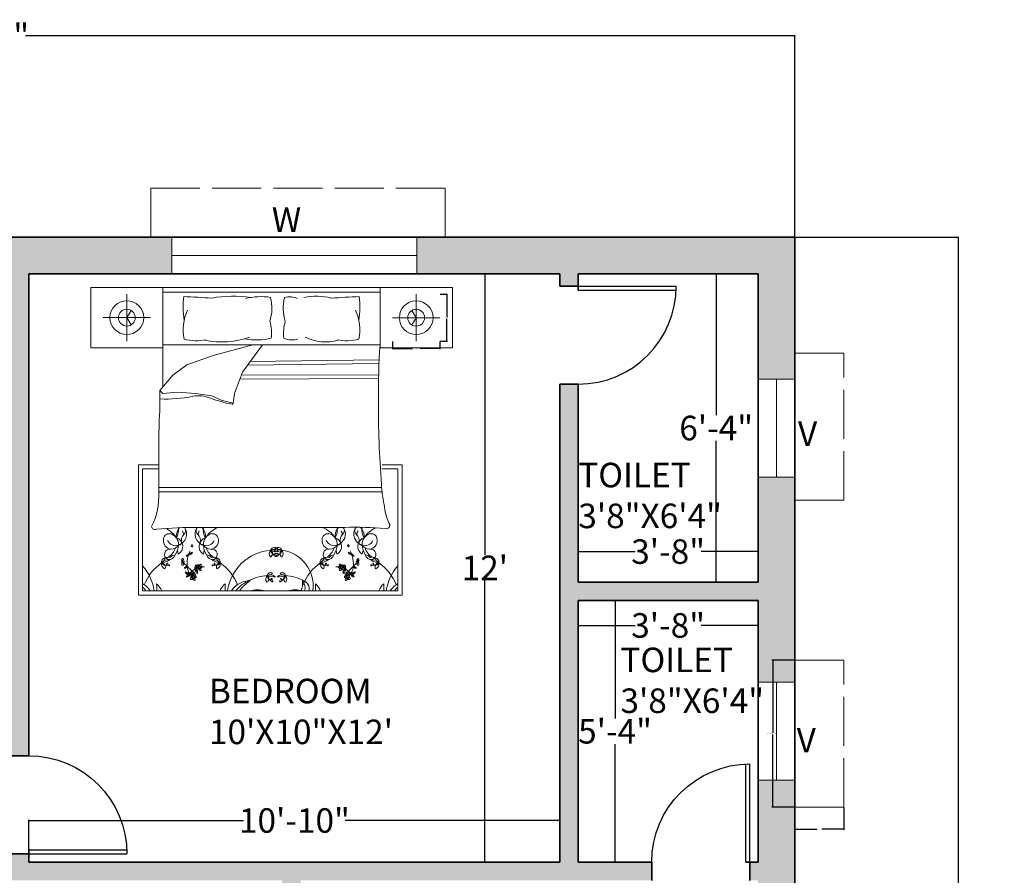
# Model space of a CAD drawing. Units: inches. Extents: x -5 to 482, y -460 to 66.
# Tile 31 of 31: x 241 to 482, y -143 to 66. Entities that reach past the tile are written whole.
import ezdxf

# ---------------------------------------------------------------- set-up
doc = ezdxf.new("R2010")
doc.units = ezdxf.units.IN
doc.header["$MEASUREMENT"] = 0
doc.linetypes.add('ACAD_ISO02W100', pattern=[15, 12, -3])
for name, color, linetype, lineweight in [('A-ANNO-DIMS', 2, 'Continuous', 18), ('A-ANNO-TEXT', 7, 'Continuous', 18), ('A-AREA-IDEN', 7, 'Continuous', 18), ('A-DOOR', 3, 'Continuous', 25), ('A-FURN', 8, 'Continuous', 18), ('A-GLAZ', 4, 'Continuous', 18), ('A-GLAZ-OVHD', 4, 'ACAD_ISO02W100', 13), ('A-WALL', 7, 'Continuous', 35), ('A-WALL-PATT', 152, 'Continuous', 13)]:
    doc.layers.add(name, color=color, linetype=linetype, lineweight=lineweight)
doc.styles.get("Standard").update_dxf_attribs({"font": 'arial.ttf'})
doc.dimstyles.get("Standard").update_dxf_attribs({"dimtxt": 0.18, "dimasz": 0.18, "dimexe": 0.18, "dimexo": 0.0625, "dimgap": 0.09, "dimtad": 0, "dimtih": 1, "dimtoh": 1, "dimdec": 0, "dimzin": 0, "dimdsep": 46, "dimlunit": 3, "dimtxsty": 'Standard', "dimcen": 0.09, "dimadec": 0, "dimazin": 0, "dimtfac": 1, "dimtdec": 0, "dimtofl": 0, "dimtmove": 0, "dimatfit": 3, "dimfxl": 1, "dimtolj": 1, "dimtzin": 0, "dimarcsym": 0})

# ---------------------------------------------------------------- blocks, each defined once
blk = doc.blocks.new('*D3')
at = {"layer": 'A-ANNO-DIMS', "color": 0, "lineweight": -2, "transparency": 16777216}
for p, q in [((32.88, 13.21), (32.88, 62.61)), ((33.06, 62.43), (221.23, 62.43)), ((430.2, 62.43), (242.02, 62.43)), ((430.38, 13.21), (430.38, 62.61))]:
    blk.add_line(p, q, dxfattribs=at)
at = {"layer": 'A-ANNO-DIMS', "color": 0, "transparency": 16777216}
for points in [[(33.06, 62.46), (33.06, 62.4), (32.88, 62.43)], [(430.2, 62.46), (430.2, 62.4), (430.38, 62.43)]]:
    blk.add_solid(points, dxfattribs=at)
at = {"layer": 'Defpoints', "color": 0, "transparency": 16777216}
for p in [(430.38, 62.43), (32.88, 13.15), (430.38, 13.15)]:
    blk.add_point(p, dxfattribs=at)
at = {"layer": 'A-ANNO-DIMS', "color": 0, "transparency": 16777216, "insert": (231.63, 62.43), "char_height": 6, "attachment_point": 5}
blk.add_mtext('\\A1;33\'-2"', dxfattribs=at)
blk = doc.blocks.new('*D4')
at = {"layer": 'A-ANNO-DIMS', "color": 0, "lineweight": -2, "transparency": 16777216}
for p, q in [((430.44, 13.15), (470.55, 13.15)), ((470.37, 12.97), (470.37, -201.19)), ((470.37, -421.67), (470.37, -207.5)), ((430.44, -421.85), (470.55, -421.85))]:
    blk.add_line(p, q, dxfattribs=at)
at = {"layer": 'A-ANNO-DIMS', "color": 0, "transparency": 16777216}
for points in [[(470.34, 12.97), (470.4, 12.97), (470.37, 13.15)], [(470.34, -421.67), (470.4, -421.67), (470.37, -421.85)]]:
    blk.add_solid(points, dxfattribs=at)
at = {"layer": 'Defpoints', "color": 0, "transparency": 16777216}
for p in [(430.38, 13.15), (430.38, -421.85), (470.37, -421.85)]:
    blk.add_point(p, dxfattribs=at)
at = {"layer": 'A-ANNO-DIMS', "color": 0, "transparency": 16777216, "insert": (470.37, -204.35), "char_height": 6, "attachment_point": 5}
blk.add_mtext('\\A1;36\'-3"', dxfattribs=at)
blk = doc.blocks.new('*D9')
at = {"layer": 'A-ANNO-DIMS', "color": 0, "lineweight": -2, "transparency": 16777216}
for p, q in [((242.88, -137.79), (242.88, -129.51)), ((243.06, -129.69), (295.43, -129.69)), ((372.7, -129.69), (320.32, -129.69)), ((372.88, -129.63), (372.88, -129.51))]:
    blk.add_line(p, q, dxfattribs=at)
at = {"layer": 'A-ANNO-DIMS', "color": 0, "transparency": 16777216}
for points in [[(243.06, -129.66), (243.06, -129.72), (242.88, -129.69)], [(372.7, -129.66), (372.7, -129.72), (372.88, -129.69)]]:
    blk.add_solid(points, dxfattribs=at)
at = {"layer": 'Defpoints', "color": 0, "transparency": 16777216}
for p in [(372.88, -129.69), (372.88, -129.69), (242.88, -137.85)]:
    blk.add_point(p, dxfattribs=at)
at = {"layer": 'A-ANNO-DIMS', "color": 0, "transparency": 16777216, "insert": (307.88, -129.69), "char_height": 6, "attachment_point": 5}
blk.add_mtext('\\A1;10\'-10"', dxfattribs=at)
blk = doc.blocks.new('*D10')
at = {"layer": 'A-ANNO-DIMS', "color": 0, "lineweight": -2, "transparency": 16777216}
for p, q in [((355.37, 4.15), (354.32, 4.15)), ((354.5, 3.97), (354.5, -64.75)), ((354.5, -139.67), (354.5, -70.95)), ((355.37, -139.85), (354.32, -139.85))]:
    blk.add_line(p, q, dxfattribs=at)
at = {"layer": 'A-ANNO-DIMS', "color": 0, "transparency": 16777216}
for points in [[(354.47, 3.97), (354.53, 3.97), (354.5, 4.15)], [(354.47, -139.67), (354.53, -139.67), (354.5, -139.85)]]:
    blk.add_solid(points, dxfattribs=at)
at = {"layer": 'Defpoints', "color": 0, "transparency": 16777216}
for p in [(355.43, 4.15), (354.5, -139.85), (355.43, -139.85)]:
    blk.add_point(p, dxfattribs=at)
at = {"layer": 'A-ANNO-DIMS', "color": 0, "transparency": 16777216, "insert": (354.5, -67.85), "char_height": 6, "attachment_point": 5}
blk.add_mtext("\\A1;12'", dxfattribs=at)
blk = doc.blocks.new('*D11')
at = {"layer": 'A-ANNO-DIMS', "color": 0, "lineweight": -2, "transparency": 16777216}
for p, q in [((377.38, -63.79), (377.38, -63.67)), ((377.56, -63.85), (391.31, -63.85)), ((421.2, -63.85), (407.44, -63.85)), ((421.38, -63.79), (421.38, -63.67))]:
    blk.add_line(p, q, dxfattribs=at)
at = {"layer": 'A-ANNO-DIMS', "color": 0, "transparency": 16777216}
for points in [[(377.56, -63.82), (377.56, -63.88), (377.38, -63.85)], [(421.2, -63.82), (421.2, -63.88), (421.38, -63.85)]]:
    blk.add_solid(points, dxfattribs=at)
at = {"layer": 'Defpoints', "color": 0, "transparency": 16777216}
for p in [(377.38, -63.85), (421.38, -63.85), (421.38, -63.85)]:
    blk.add_point(p, dxfattribs=at)
at = {"layer": 'A-ANNO-DIMS', "color": 0, "transparency": 16777216, "insert": (399.38, -63.85), "char_height": 6, "attachment_point": 5}
blk.add_mtext('\\A1;3\'-8"', dxfattribs=at)
blk = doc.blocks.new('*D12')
at = {"layer": 'A-ANNO-DIMS', "color": 0, "lineweight": -2, "transparency": 16777216}
for p, q in [((417.62, 4.15), (410.96, 4.15)), ((411.14, 3.97), (411.14, -30.45)), ((411.14, -71.17), (411.14, -36.75)), ((417.62, -71.35), (410.96, -71.35))]:
    blk.add_line(p, q, dxfattribs=at)
at = {"layer": 'A-ANNO-DIMS', "color": 0, "transparency": 16777216}
for points in [[(411.11, 3.97), (411.17, 3.97), (411.14, 4.15)], [(411.11, -71.17), (411.17, -71.17), (411.14, -71.35)]]:
    blk.add_solid(points, dxfattribs=at)
at = {"layer": 'Defpoints', "color": 0, "transparency": 16777216}
for p in [(411.14, 4.15), (417.69, 4.15), (417.69, -71.35)]:
    blk.add_point(p, dxfattribs=at)
at = {"layer": 'A-ANNO-DIMS', "color": 0, "transparency": 16777216, "insert": (411.14, -33.6), "char_height": 6, "attachment_point": 5}
blk.add_mtext('\\A1;6\'-4"', dxfattribs=at)
blk = doc.blocks.new('*D13')
at = {"layer": 'A-ANNO-DIMS', "color": 0, "lineweight": -2, "transparency": 16777216}
for p, q in [((377.38, -81.87), (377.38, -81.75)), ((377.56, -81.93), (391.31, -81.93)), ((421.2, -81.93), (407.44, -81.93)), ((421.38, -81.87), (421.38, -81.75))]:
    blk.add_line(p, q, dxfattribs=at)
at = {"layer": 'A-ANNO-DIMS', "color": 0, "transparency": 16777216}
for points in [[(377.56, -81.9), (377.56, -81.96), (377.38, -81.93)], [(421.2, -81.9), (421.2, -81.96), (421.38, -81.93)]]:
    blk.add_solid(points, dxfattribs=at)
at = {"layer": 'Defpoints', "color": 0, "transparency": 16777216}
for p in [(377.38, -81.93), (421.38, -81.93), (421.38, -81.93)]:
    blk.add_point(p, dxfattribs=at)
at = {"layer": 'A-ANNO-DIMS', "color": 0, "transparency": 16777216, "insert": (399.38, -81.93), "char_height": 6, "attachment_point": 5}
blk.add_mtext('\\A1;3\'-8"', dxfattribs=at)
blk = doc.blocks.new('*D14')
at = {"layer": 'A-ANNO-DIMS', "color": 0, "lineweight": -2, "transparency": 16777216}
for p, q in [((382.91, -75.85), (386.56, -75.85)), ((386.38, -76.03), (386.38, -104.71)), ((386.38, -139.67), (386.38, -110.99)), ((386.44, -139.85), (386.56, -139.85))]:
    blk.add_line(p, q, dxfattribs=at)
at = {"layer": 'A-ANNO-DIMS', "color": 0, "transparency": 16777216}
for points in [[(386.35, -76.03), (386.41, -76.03), (386.38, -75.85)], [(386.35, -139.67), (386.41, -139.67), (386.38, -139.85)]]:
    blk.add_solid(points, dxfattribs=at)
at = {"layer": 'Defpoints', "color": 0, "transparency": 16777216}
for p in [(382.85, -75.85), (386.38, -75.85), (386.38, -139.85)]:
    blk.add_point(p, dxfattribs=at)
at = {"layer": 'A-ANNO-DIMS', "color": 0, "transparency": 16777216, "insert": (386.38, -107.85), "char_height": 6, "attachment_point": 5}
blk.add_mtext('\\A1;5\'-4"', dxfattribs=at)
blk = doc.blocks.new('DOOR-SWING-24IN')
for p, q in [((24, 1), (0, 1)), ((24, 0), (0, 0))]:
    blk.add_line(p, q)
blk.add_arc((24, 0), 24, 90, 180)
blk = doc.blocks.new('WIN-GLAZ-60IN')
for p, q in [((0, 9), (60, 9)), ((0, 4.5), (60, 4.5)), ((60, 0), (0, 0))]:
    blk.add_line(p, q)
blk = doc.blocks.new('VENT-GLAZ-24IN')
for p, q in [((0, 9), (24, 9)), ((0, 4.5), (24, 4.5)), ((24, 0), (0, 0))]:
    blk.add_line(p, q)
blk = doc.blocks.new('WIN-SHADE-72IN')
for p, q in [((0, 12), (72, 12)), ((0, 12), (0, 0)), ((72, 12), (72, 0))]:
    blk.add_line(p, q)
blk = doc.blocks.new('VENT-SHADE-36IN')
for p, q in [((0, 0), (0, 12)), ((36, 0), (36, 12)), ((0, 0), (36, 0))]:
    blk.add_line(p, q)
blk = doc.blocks.new('BEDSIDE-LAMP-8IN')
for p, q in [((5.79, 0), (5.79, 11.57)), ((0, 5.78), (11.57, 5.78))]:
    blk.add_line(p, q)
for points in [[(5.79, 5.78), (4.75, 7.57)], [(5.79, 5.78), (4.75, 4)]]:
    blk.add_lwpolyline(points)
for radius in [4.13, 2.07]:
    blk.add_circle((5.79, 5.78), radius)
blk = doc.blocks.new('*D51')
at = {"layer": 'A-ANNO-DIMS', "color": 0, "lineweight": -2, "transparency": 16777216}
for p, q in [((430.31, -90.42), (424.8, -90.42)), ((424.98, -90.6), (424.98, -108.23)), ((424.98, -126.24), (424.98, -108.6)), ((430.31, -126.42), (424.8, -126.42))]:
    blk.add_line(p, q, dxfattribs=at)
at = {"layer": 'A-ANNO-DIMS', "color": 0, "transparency": 16777216}
for points in [[(424.95, -90.6), (425.01, -90.6), (424.98, -90.42)], [(424.95, -126.24), (425.01, -126.24), (424.98, -126.42)]]:
    blk.add_solid(points, dxfattribs=at)
at = {"layer": 'Defpoints', "color": 0, "transparency": 16777216}
for p in [(424.98, -90.42), (430.38, -90.42), (430.38, -126.42)]:
    blk.add_point(p, dxfattribs=at)
at = {"layer": 'A-ANNO-DIMS', "color": 0, "transparency": 16777216, "insert": (424.98, -108.42), "char_height": 0.18, "attachment_point": 5}
blk.add_mtext('\\A1;VENT SHADE 3\'-0" TYP.', dxfattribs=at)
blk = doc.blocks.new('*D52')
at = {"layer": 'A-ANNO-DIMS', "color": 0, "lineweight": -2, "transparency": 16777216}
for p, q in [((430.38, -126.48), (430.38, -132)), ((442.38, -126.48), (442.38, -132)), ((430.56, -131.82), (435.75, -131.82)), ((442.2, -131.82), (437.01, -131.82))]:
    blk.add_line(p, q, dxfattribs=at)
at = {"layer": 'A-ANNO-DIMS', "color": 0, "transparency": 16777216}
for points in [[(430.56, -131.79), (430.56, -131.85), (430.38, -131.82)], [(442.2, -131.79), (442.2, -131.85), (442.38, -131.82)]]:
    blk.add_solid(points, dxfattribs=at)
at = {"layer": 'Defpoints', "color": 0, "transparency": 16777216}
for p in [(430.38, -126.42), (442.38, -126.42), (430.38, -131.82)]:
    blk.add_point(p, dxfattribs=at)
at = {"layer": 'A-ANNO-DIMS', "color": 0, "transparency": 16777216, "insert": (436.38, -131.82), "char_height": 0.18, "attachment_point": 5}
blk.add_mtext('\\A1;1\'-0" TYP.', dxfattribs=at)
blk = doc.blocks.new('*D55')
at = {"layer": 'A-ANNO-DIMS', "color": 0, "lineweight": -2, "transparency": 16777216}
for p, q in [((343.54, -0.8), (345.39, -0.8)), ((345.21, -0.98), (345.21, -6.4)), ((345.21, -12.19), (345.21, -6.77)), ((343.54, -12.37), (345.39, -12.37))]:
    blk.add_line(p, q, dxfattribs=at)
at = {"layer": 'A-ANNO-DIMS', "color": 0, "transparency": 16777216}
for points in [[(345.18, -0.98), (345.24, -0.98), (345.21, -0.8)], [(345.18, -12.19), (345.24, -12.19), (345.21, -12.37)]]:
    blk.add_solid(points, dxfattribs=at)
at = {"layer": 'Defpoints', "color": 0, "transparency": 16777216}
for p in [(343.48, -0.8), (345.21, -0.8), (343.48, -12.37)]:
    blk.add_point(p, dxfattribs=at)
at = {"layer": 'A-ANNO-DIMS', "color": 0, "transparency": 16777216, "insert": (345.21, -6.58), "char_height": 0.18, "attachment_point": 5}
blk.add_mtext('\\A1;BEDSIDE LAMP 0\'-11 1/2" TYP.', dxfattribs=at)
blk = doc.blocks.new('*D56')
at = {"layer": 'A-ANNO-DIMS', "color": 0, "lineweight": -2, "transparency": 16777216}
for p, q in [((331.91, -12.43), (331.91, -14.28)), ((332.09, -14.1), (336.78, -14.1)), ((343.3, -14.1), (338.61, -14.1)), ((343.48, -12.43), (343.48, -14.28))]:
    blk.add_line(p, q, dxfattribs=at)
at = {"layer": 'A-ANNO-DIMS', "color": 0, "transparency": 16777216}
for points in [[(332.09, -14.07), (332.09, -14.13), (331.91, -14.1)], [(343.3, -14.07), (343.3, -14.13), (343.48, -14.1)]]:
    blk.add_solid(points, dxfattribs=at)
at = {"layer": 'Defpoints', "color": 0, "transparency": 16777216}
for p in [(331.91, -12.37), (343.48, -12.37), (343.48, -14.1)]:
    blk.add_point(p, dxfattribs=at)
at = {"layer": 'A-ANNO-DIMS', "color": 0, "transparency": 16777216, "insert": (337.69, -14.1), "char_height": 0.18, "attachment_point": 5}
blk.add_mtext('\\A1;0\'-11 1/2" TYP.', dxfattribs=at)

msp = doc.modelspace()

# ---------------------------------------------------------------- hatches: boundary and pattern name
at = {"layer": 'A-WALL-PATT'}
h = msp.add_hatch(color=256, dxfattribs=at)
h.dxf.hatch_style = 1
h.paths.add_polyline_path([(149.38, -412.85), (144.38, -412.85), (144.38, -283.85), (144.38, -279.35), (133.88, -279.35), (133.88, -283.85), (139.88, -283.85), (139.88, -412.85), (133.51, -412.85), (133.51, -413.92), (102.65, -413.92), (102.65, -421.02), (133.51, -421.02), (133.51, -421.85), (149.38, -421.85)])
h.paths.add_polyline_path([(226.05, -412.85), (218.88, -412.85), (218.88, -350.85), (262.88, -350.85), (262.88, -386.85), (267.38, -386.85), (267.38, -283.85), (270.38, -283.85), (270.38, -279.35), (244.88, -279.35), (244.88, -283.85), (262.88, -283.85), (262.88, -346.35), (218.88, -346.35), (218.88, -283.85), (220.88, -283.85), (220.88, -279.35), (214.38, -279.35), (214.38, -283.85), (214.38, -412.85), (209.38, -412.85), (209.38, -421.85), (226.05, -421.85)])
h.paths.add_polyline_path([(315.81, -412.85), (250.05, -412.85), (250.05, -421.85), (315.81, -421.85)])
h.paths.add_polyline_path([(430.38, -378.35), (421.38, -378.35), (421.38, -412.85), (375.81, -412.85), (375.81, -421.85), (430.38, -421.85)])
h.paths.add_polyline_path([(78.69, -413.92), (47.68, -413.92), (47.68, -412.85), (41.88, -412.85), (41.88, -283.85), (109.88, -283.85), (109.88, -279.35), (41.88, -279.35), (41.88, -241.85), (32.88, -241.85), (32.88, -421.85), (47.68, -421.85), (47.68, -421.02), (78.69, -421.02)])
h.paths.add_polyline_path([(41.88, -144.35), (154.38, -144.35), (154.38, -137.85), (149.88, -137.85), (149.88, -139.85), (41.88, -139.85), (41.88, -97.85), (32.88, -97.85), (32.88, -181.85), (41.88, -181.85)])
h.paths.add_polyline_path([(430.38, -241.85), (421.38, -241.85), (421.38, -279.35), (309.38, -279.35), (309.38, -170.35), (304.88, -170.35), (304.88, -279.35), (294.38, -279.35), (294.38, -283.85), (421.38, -283.85), (421.38, -318.35), (430.38, -318.35)])
h.paths.add_polyline_path([(430.38, -119.85), (421.38, -119.85), (421.38, -139.85), (419.38, -139.85), (419.38, -144.35), (421.38, -144.35), (421.38, -181.85), (430.38, -181.85)])
h.paths.add_polyline_path([(395.38, -139.85), (377.38, -139.85), (377.38, -75.85), (421.38, -75.85), (421.38, -95.85), (430.38, -95.85), (430.38, -45.6), (421.38, -45.6), (421.38, -71.35), (377.38, -71.35), (377.38, -22.85), (372.88, -22.85), (372.88, -139.85), (242.88, -139.85), (242.88, -137.85), (238.38, -137.85), (238.38, -144.35), (304.88, -144.35), (304.88, -146.35), (309.38, -146.35), (309.38, -144.35), (395.38, -144.35)])
h.paths.add_polyline_path([(65.88, 13.15), (32.88, 13.15), (32.88, -37.85), (41.88, -37.85), (41.88, 4.15), (65.88, 4.15)])
h.paths.add_polyline_path([(166.38, 13.15), (125.88, 13.15), (125.88, 4.15), (149.88, 4.15), (149.88, -113.85), (154.38, -113.85), (154.38, 4.15), (166.38, 4.15)])
h.paths.add_polyline_path([(277.88, 13.15), (226.38, 13.15), (226.38, 4.15), (238.38, 4.15), (238.38, -113.85), (242.88, -113.85), (242.88, 4.15), (277.88, 4.15)])
h.paths.add_polyline_path([(430.38, 13.15), (337.88, 13.15), (337.88, 4.15), (372.88, 4.15), (372.88, 1.15), (377.38, 1.15), (377.38, 4.15), (421.38, 4.15), (421.38, -21.6), (430.38, -21.6)])

# ---------------------------------------------------------------- linework, layer by layer
at = {"layer": 'A-FURN'}
for p, q in [((258.01, 0.8), (346.55, 0.8)), ((275.71, 0.8), (275.71, -23.51)), ((328.84, -0.34), (275.71, -0.34)), ((275.71, -13.2), (328.84, -13.2)), ((288.01, -15.83), (297.67, -13.2)), ((300.04, -13.2), (295.19, -19.95)), ((281.56, -18.16), (288.01, -15.83)), ((278.15, -20.67), (281.56, -18.16)), ((328.57, -17.78), (296.42, -18.24)), ((328.6, -16.87), (297.08, -17.32)), ((274.92, -24.43), (278.15, -20.67)), ((295.19, -19.95), (293.21, -25.15)), ((328.53, -21.48), (294.55, -21.62)), ((328.52, -20.57), (294.9, -20.7)), ((275.64, -25.15), (274.92, -24.43)), ((279.23, -24.79), (275.64, -25.15)), ((283.71, -25.15), (279.23, -24.79)), ((287.65, -25.68), (283.71, -25.15)), ((289.99, -26.76), (287.65, -25.68)), ((293.21, -25.15), (292.86, -27.48)), ((292.86, -27.48), (289.99, -26.76)), ((269.69, -42.61), (274.7, -42.61)), ((269.69, -74.5), (269.69, -42.61)), ((329.33, -42.61), (334.24, -42.61)), ((334.24, -42.61), (334.24, -74.5)), ((274.7, -43.63), (270.72, -43.63)), ((270.72, -43.63), (270.72, -73.48)), ((333.22, -43.63), (329.31, -43.63)), ((333.22, -73.48), (333.22, -43.63)), ((329.24, -48.13), (274.69, -48.13)), ((329.33, -49.23), (274.69, -49.23)), ((320.25, -57.93), (284.3, -57.93)), ((279.44, -64.5), (279.25, -63.5)), ((285.63, -64.5), (285.83, -63.5)), ((318.3, -64.5), (318.11, -63.5)), ((324.49, -64.5), (324.69, -63.5)), ((334.24, -74.5), (269.69, -74.5)), ((270.72, -73.48), (333.22, -73.48))]:
    msp.add_line(p, q, dxfattribs=at)
for points in [[(275.71, -13.96), (258.01, -13.96), (258.01, 0.8)], [(328.84, 0.8), (328.84, -13.96), (346.55, -13.96), (346.55, 0.8)]]:
    msp.add_lwpolyline(points, dxfattribs=at)
for points in [[(280.8, -1.41, 0.074897), (280.91, -7.19, -0.472817)], [(301.86, -7.52, 0.14099), (302.04, -1.62, 0.235245)], [(305.64, -7.52, -0.14099), (305.47, -1.62, -0.235245)], [(323.75, -1.41, -0.074897), (323.65, -7.19, 0.472817)], [(274.74, -32.54, 0.001242), (274.69, -49.34, -0.127202), (272.92, -57.71)], [(329.22, -47.43, 0.056112), (329.86, -52.3, 0.095341), (331.1, -57)]]:
    msp.add_lwpolyline(points, format="xyb", dxfattribs=at)
for centre in [(284.56, -67.71), (319.38, -67.71), (283.08, -70.09), (320.85, -70.09)]:
    msp.add_circle(centre, 0.225, dxfattribs=at)
for centre, radius, start, end in [((329.6, 841.22), 844.04, 266.68521, 267.14978), ((292.93, -33.45), 32.11, 82.2196, 99.497), ((299.71, -17.22), 15.78, 81.5249, 103.96), ((306.68, -5.83), 4.38, 63.3437, 106.1026), ((313.25, -16.9), 15.57, 76.3427, 101.1841), ((274.95, 841.22), 844.04, 272.85022, 273.31479), ((292.08, -9.52), 11.41, 155.1316, 191.7583), ((312.47, -9.52), 11.41, 348.2417, 24.8684), ((291.43, -10.48), 10.85, 354.0129, 15.8293), ((316.08, -10.48), 10.85, 164.1707, 185.9871), ((283.96, -0.37), 11.87, 255.1039, 281.0369), ((290.2, 8.06), 20.58, 258.0397, 289.2615), ((298.54, 3.57), 15.61, 259.8617, 283.6238), ((307.27, -7.35), 4.69, 245.0183, 288.5407), ((315.47, -1.25), 11.27, 243.8761, 286.1746), ((320.6, -0.37), 11.87, 258.9631, 284.8961), ((487.57, -24.02), 159.1, 176.1, 180.9282), ((193.74, -26.63), 81.21, 355.8294, 1.553), ((276.44, 6.92), 33.42, 267.4519, 281.3392), ((284.42, -32.91), 7.21, 66.2616, 101.3392), ((299, 5.98), 34.34, 250.1194, 259.3383), ((292.65, -27.55), 0.214, 268.8623, 19.7536), ((536, -29.8), 207.53, 179.1145, 184.8735), ((273.73, -57.65), 0.817, 183.98, 297.3412), ((330.43, -57.45), 0.807, 246.5219, 33.8264), ((283.25, -150.1), 92.17, 89.3433, 95.6887), ((277.29, -60.95), 1.49, 84.4856, 181.0538), ((273.39, -64.17), 6.7, 33.6671, 63.2997), ((276.83, -62.05), 2.66, 355.2933, 76.921), ((282.37, -60.18), 3.41, 145.785, 184.7304), ((275.85, -58.59), 3.67, 328.8218, 9.1554), ((280.39, -58.91), 1.07, 120.0293, 142.325), ((278.69, -59.54), 2.82, 289.2822, 29.1751), ((282.02, -61.05), 1.82, 131.5653, 195.1471), ((278.26, -60.05), 2.55, 7.436, 29.9149), ((279.94, -58.7), 1.32, 311.5653, 23.8354), ((280.39, -58.91), 1.07, 44.4517, 63.558), ((286.39, -59.54), 2.82, 150.8249, 250.7178), ((285.14, -58.7), 1.32, 156.1646, 228.4347), ((284.69, -58.91), 1.07, 113.229, 135.5483), ((283.05, -61.05), 1.82, 344.8529, 48.4347), ((286.81, -60.05), 2.55, 150.0851, 172.564), ((284.69, -58.91), 1.07, 37.675, 66.7144), ((282.71, -60.18), 3.41, 355.2696, 34.215), ((289.23, -58.59), 3.67, 169.7133, 211.1782), ((288.24, -62.05), 2.66, 103.079, 184.7067), ((291.69, -64.17), 6.7, 111.4941, 146.3329), ((287.78, -60.95), 1.49, 358.9462, 95.5144), ((316.15, -60.95), 1.49, 84.4856, 181.0538), ((312.25, -64.17), 6.7, 33.6671, 68.5059), ((315.69, -62.05), 2.66, 355.2933, 76.921), ((321.23, -60.18), 3.41, 145.785, 184.7304), ((314.71, -58.59), 3.67, 328.8218, 10.2867), ((319.25, -58.91), 1.07, 113.2856, 142.325), ((317.55, -59.54), 2.82, 289.2822, 29.1751), ((320.88, -61.05), 1.82, 131.5653, 195.1471), ((317.12, -60.05), 2.55, 7.436, 29.9149), ((319.25, -58.91), 1.07, 44.4517, 66.7144), ((318.8, -58.7), 1.32, 311.5653, 23.8354), ((322.96, -144.05), 86.16, 85.2402, 91.8035), ((325.25, -59.54), 2.82, 150.8249, 250.7178), ((324, -58.7), 1.32, 156.1646, 228.4347), ((323.55, -58.91), 1.07, 106.6343, 135.5483), ((321.91, -61.05), 1.82, 344.8529, 48.4347), ((325.67, -60.05), 2.55, 150.0851, 172.564), ((323.55, -58.91), 1.07, 37.675, 72.5814), ((321.57, -60.18), 3.41, 355.2696, 34.215), ((328.09, -58.59), 3.67, 169.249, 211.1782), ((327.1, -62.05), 2.66, 103.079, 184.7067), ((330.55, -64.17), 6.7, 113.6453, 146.3329), ((326.64, -60.95), 1.49, 358.9462, 95.5144), ((277.91, -61.16), 2.12, 174.9449, 262.8857), ((278.74, -60.36), 2.05, 201.5819, 291.4221), ((277.54, -60.69), 2.57, 272.3591, 324.0401), ((274.75, -61.98), 4.75, 326.2883, 356.5076), ((278.35, -62.59), 2.2, 299.9085, 73.1337), ((282.37, -60.18), 3.41, 212.7011, 216.3445), ((279.74, -61.67), 0.55, 257.3041, 15.1471), ((282.79, -62.5), 0.171, 102.7051, 280.4384), ((282.77, -62.4), 0.277, 280.4384, 100.4136), ((286.73, -62.59), 2.2, 106.8663, 240.0915), ((285.34, -61.67), 0.55, 164.8529, 282.6959), ((282.71, -60.18), 3.41, 323.6555, 327.2989), ((287.54, -60.69), 2.57, 215.9599, 267.6409), ((286.34, -60.36), 2.05, 248.5779, 338.4181), ((290.33, -61.98), 4.75, 183.4924, 213.7117), ((287.17, -61.16), 2.12, 277.1143, 5.0551), ((316.77, -61.16), 2.12, 174.9449, 262.8857), ((317.6, -60.36), 2.05, 201.5819, 291.4221), ((316.4, -60.69), 2.57, 272.3591, 324.0401), ((313.61, -61.98), 4.75, 326.2883, 356.5076), ((317.21, -62.59), 2.2, 299.9085, 73.1337), ((321.23, -60.18), 3.41, 212.7011, 216.3445), ((318.6, -61.67), 0.55, 257.3041, 15.1471), ((321.16, -62.4), 0.277, 79.5864, 259.5616), ((321.14, -62.5), 0.171, 259.5616, 77.2949), ((325.59, -62.59), 2.2, 106.8663, 240.0915), ((324.2, -61.67), 0.55, 164.8529, 282.6959), ((321.57, -60.18), 3.41, 323.6555, 327.2989), ((326.4, -60.69), 2.57, 215.9599, 267.6409), ((325.2, -60.36), 2.05, 248.5779, 338.4181), ((329.19, -61.98), 4.75, 183.4924, 213.7117), ((326.03, -61.16), 2.12, 277.1143, 5.0551), ((277.42, -64.57), 1.33, 80.264, 250.8688), ((274.78, -61.65), 4.18, 301.2614, 341.7045), ((277.1, -64.17), 1.66, 265.969, 344.3045), ((278.89, -66.38), 1.77, 96.1662, 141.5825), ((281.81, -65.14), 0.465, 101.3256, 154.4621), ((281.15, -63.56), 1.4, 280.2588, 300.656), ((281.47, -62.44), 2.5, 268.3264, 277.1302), ((288.93, -66.96), 7.33, 163.5842, 183.8277), ((280.84, -63.56), 1.42, 308.2101, 316.3071), ((281.72, -64.5), 0.425, 278.3432, 4.2869), ((281.48, -64.13), 0.742, 300.656, 332.6341), ((282.04, -64.62), 0.18, 55.7657, 157.4417), ((288.93, -66.96), 7.33, 153.0032, 159.8941), ((282.32, -64.45), 0.18, 84.3784, 186.0543), ((282.15, -63.73), 0.742, 269.1859, 301.164), ((282.37, -64.11), 0.425, 237.5332, 323.4768), ((281.96, -62.9), 1.42, 285.5129, 293.6099), ((281.81, -63.16), 1.4, 301.164, 321.5612), ((282.89, -64.5), 0.465, 87.3579, 140.4944), ((280.67, -62.92), 2.5, 324.6898, 333.4936), ((290.29, -61.65), 4.18, 198.2955, 238.7386), ((286.19, -66.38), 1.77, 38.4175, 83.8338), ((287.98, -64.17), 1.66, 195.6955, 274.031), ((287.66, -64.57), 1.33, 289.1312, 99.736), ((302.97, -75.04), 11.56, 94.4623, 172.255), ((303.02, -64.37), 1.28, 137.7873, 219.1145), ((301.56, -64.33), 0.966, 298.5391, 58.3627), ((302.99, -63.78), 0.959, 63.0274, 163.8037), ((302.02, -61.53), 1.97, 271.4585, 315.3727), ((302.82, -65.17), 1.83, 45.5411, 114.3101), ((304.49, -55.79), 8.09, 252.593, 267.2582), ((303.01, -63.54), 0.946, 177.7585, 283.852), ((304.83, -62.56), 2.92, 198.9159, 238.011), ((304.07, -65.17), 1.83, 65.6899, 134.4589), ((302.4, -55.79), 8.09, 272.7418, 287.407), ((303.21, -64.34), 0.125, 283.852, 219.9245), ((303.36, -64.92), 0.144, 238.011, 71.5592), ((303.38, -64.85), 0.0698, 71.5592, 188.0167), ((303.53, -64.92), 0.144, 108.4408, 301.989), ((303.9, -63.78), 0.959, 16.1963, 116.9726), ((304.87, -61.53), 1.97, 224.6273, 268.5415), ((303.51, -64.85), 0.0698, 351.9833, 108.4408), ((303.67, -64.29), 0.0754, 320.1909, 256.0209), ((302.06, -62.56), 2.92, 301.989, 341.0841), ((303.88, -63.54), 0.946, 256.148, 2.2415), ((305.33, -64.33), 0.966, 121.6373, 241.4609), ((303.87, -64.37), 1.28, 320.8855, 42.2127), ((303.55, -72.37), 8.95, 352.8636, 81.8197), ((316.28, -64.57), 1.33, 80.264, 250.8688), ((313.64, -61.65), 4.18, 301.2614, 341.7045), ((315.96, -64.17), 1.66, 265.969, 344.3045), ((317.75, -66.38), 1.77, 96.1662, 141.5825), ((322.13, -63.16), 1.4, 218.4388, 238.836), ((321.05, -64.5), 0.465, 39.5056, 92.6421), ((323.26, -62.92), 2.5, 206.5064, 215.3102), ((321.57, -64.11), 0.425, 216.5232, 302.4668), ((321.79, -63.73), 0.742, 238.836, 270.8141), ((321.98, -62.9), 1.42, 246.3901, 254.4871), ((315.01, -66.96), 7.33, 20.1059, 26.9968), ((321.62, -64.45), 0.18, 353.9457, 95.6216), ((321.9, -64.62), 0.18, 22.5583, 124.2343), ((322.22, -64.5), 0.425, 175.7131, 261.6568), ((322.46, -64.13), 0.742, 207.3659, 239.344), ((315.01, -66.96), 7.33, 356.1723, 16.4158), ((323.09, -63.56), 1.42, 223.6929, 231.7899), ((322.79, -63.56), 1.4, 239.344, 259.7412), ((322.47, -62.44), 2.5, 262.8698, 271.6736), ((322.12, -65.14), 0.465, 25.5379, 78.6744), ((329.15, -61.65), 4.18, 198.2955, 238.7386), ((326.84, -64.17), 1.66, 195.6955, 274.031), ((325.05, -66.38), 1.77, 38.4175, 83.8338), ((326.52, -64.57), 1.33, 289.1312, 99.736), ((262.11, -75.04), 11.56, 7.745, 41.8856), ((281.89, -76.18), 11.56, 124.3865, 158.5908), ((276.29, -66.41), 0.959, 92.9516, 193.728), ((276.62, -66.91), 1.28, 167.7115, 249.0387), ((274.33, -64.95), 1.97, 301.3827, 345.2969), ((276.85, -67.7), 1.83, 75.4653, 144.2343), ((273.61, -58.74), 8.09, 282.5173, 297.1824), ((275.33, -67.6), 0.966, 328.4633, 88.2869), ((277.29, -64.43), 2.92, 228.8402, 267.9352), ((276.2, -66.2), 0.946, 207.6827, 313.7762), ((277.15, -66.01), 0.814, 63.9755, 143.2681), ((276.77, -66.79), 0.125, 313.7762, 249.7183), ((277.17, -67.14), 0.0698, 101.4834, 217.9409), ((277.19, -67.21), 0.144, 267.9352, 101.4834), ((280.5, -66.02), 0.376, 101.5637, 142.6358), ((280.19, -66.37), 0.225, 273.2768, 86.7232), ((280.5, -66.79), 0.372, 217.7621, 259.0403), ((280.45, -66.16), 0.215, 91.1081, 181.8675), ((280.9, -66.29), 0.685, 203.4276, 227.6104), ((280.68, -66.59), 0.466, 80.3487, 133.6538), ((280.6, -66.2), 0.369, 229.7889, 317.6792), ((280.2, -65.72), 0.542, 288.7263, 352.5032), ((280.18, -66.98), 0.524, 355.053, 68.3618), ((280.59, -67.07), 0.738, 83.0852, 105.7171), ((280.57, -65.75), 0.174, 345.2356, 144.9248), ((280.53, -67.01), 0.173, 232.4737, 355.053), ((275.48, -73.2), 8.41, 43.1541, 52.0459), ((280.73, -66.32), 0.194, 317.6792, 80.3487), ((281.19, -67.48), 0.425, 278.3432, 4.2869), ((280.95, -67.11), 0.742, 300.656, 332.6341), ((281.51, -67.6), 0.18, 55.7657, 157.4417), ((285.28, -67.14), 3.68, 184.756, 209.2041), ((290.57, -59.31), 12.1, 222.2412, 232.1744), ((282.83, -67.37), 1.03, 304.5369, 16.3699), ((284.26, -67.66), 0.727, 127.3105, 187.9252), ((283.26, -67.58), 0.747, 355.0106, 41.658), ((284.31, -67.39), 0.307, 126.1046, 271.4281), ((284.28, -67.31), 0.221, 353.7526, 131.7054), ((284.07, -67.57), 0.31, 0.0645, 61.1507), ((284.14, -67.31), 0.355, 311.8413, 355.7877), ((284.87, -67.36), 0.376, 101.5637, 176.365), ((284.82, -67.5), 0.215, 91.1081, 181.8675), ((285.05, -67.93), 0.466, 80.3487, 133.6538), ((284.57, -67.06), 0.542, 288.7263, 352.5032), ((284.94, -67.09), 0.174, 345.2356, 144.9248), ((285.1, -67.66), 0.194, 317.6792, 80.3487), ((287.93, -66.01), 0.814, 36.7319, 116.0245), ((287.89, -67.21), 0.144, 78.5166, 272.0648), ((288.23, -67.7), 1.83, 35.7657, 104.5347), ((291.47, -58.74), 8.09, 242.8176, 257.4827), ((287.79, -64.43), 2.92, 272.0648, 311.1598), ((287.9, -67.14), 0.0698, 322.0591, 78.5166), ((288.88, -66.2), 0.946, 226.2238, 332.3173), ((288.32, -66.74), 0.0754, 290.2667, 226.2271), ((289.74, -67.6), 0.966, 91.7131, 211.5367), ((288.78, -66.41), 0.959, 346.272, 87.0484), ((290.74, -64.95), 1.97, 194.7031, 238.6173), ((288.46, -66.91), 1.28, 290.9613, 12.2885), ((283.18, -76.18), 11.56, 21.4092, 55.6135), ((320.75, -76.18), 11.56, 124.3865, 158.5908), ((315.15, -66.41), 0.959, 92.9516, 193.728), ((315.48, -66.91), 1.28, 167.7115, 249.0387), ((313.19, -64.95), 1.97, 301.3827, 345.2969), ((315.71, -67.7), 1.83, 75.4653, 144.2343), ((312.47, -58.74), 8.09, 282.5173, 297.1824), ((315.06, -66.2), 0.946, 207.6827, 313.7762), ((316.15, -64.43), 2.92, 228.8402, 267.9352), ((314.19, -67.6), 0.966, 328.4633, 88.2869), ((316.01, -66.01), 0.814, 63.9755, 143.2681), ((315.63, -66.79), 0.125, 313.7762, 249.7183), ((316.03, -67.14), 0.0698, 101.4834, 217.9409), ((316.05, -67.21), 0.144, 267.9352, 101.4834), ((318.84, -67.66), 0.194, 99.6513, 222.3208), ((318.89, -67.93), 0.466, 46.3462, 99.6513), ((319, -67.09), 0.174, 35.0752, 194.7644), ((319.37, -67.06), 0.542, 187.4968, 251.2737), ((319.11, -67.5), 0.215, 358.1325, 88.8919), ((319.07, -67.36), 0.376, 3.635, 78.4363), ((319.66, -67.31), 0.221, 48.2946, 186.2474), ((319.79, -67.31), 0.355, 184.2123, 228.1587), ((319.87, -67.57), 0.31, 118.8493, 179.9355), ((319.63, -67.39), 0.307, 268.5719, 53.8954), ((320.68, -67.58), 0.747, 138.342, 184.9894), ((321.1, -67.37), 1.03, 163.6301, 235.4631), ((319.68, -67.66), 0.727, 352.0748, 52.6895), ((313.37, -59.31), 12.1, 307.8256, 317.7588), ((318.66, -67.14), 3.68, 330.7959, 355.244), ((328.46, -73.2), 8.41, 127.9541, 136.8459), ((322.43, -67.6), 0.18, 22.5583, 124.2343), ((322.75, -67.48), 0.425, 175.7131, 261.6568), ((322.98, -67.11), 0.742, 207.3659, 239.344), ((323.21, -66.32), 0.194, 99.6513, 222.3208), ((323.34, -66.2), 0.369, 222.3208, 310.2111), ((323.26, -66.59), 0.466, 46.3462, 99.6513), ((323.37, -65.75), 0.174, 35.0752, 194.7644), ((323.74, -65.72), 0.542, 187.4968, 251.2737), ((323.76, -66.98), 0.524, 111.6382, 184.947), ((323.41, -67.01), 0.173, 184.947, 307.5263), ((323.35, -67.07), 0.738, 74.2829, 96.9148), ((323.49, -66.16), 0.215, 358.1325, 88.8919), ((323.04, -66.29), 0.685, 312.3896, 336.5724), ((323.44, -66.02), 0.376, 37.3642, 78.4363), ((323.44, -66.79), 0.372, 280.9597, 322.2379), ((323.75, -66.37), 0.225, 93.2768, 266.7232), ((326.79, -66.01), 0.814, 36.7319, 116.0245), ((326.75, -67.21), 0.144, 78.5166, 272.0648), ((327.09, -67.7), 1.83, 35.7657, 104.5347), ((330.33, -58.74), 8.09, 242.8176, 257.4827), ((326.65, -64.43), 2.92, 272.0648, 311.1598), ((326.76, -67.14), 0.0698, 322.0591, 78.5166), ((327.74, -66.2), 0.946, 226.2238, 332.3173), ((327.18, -66.74), 0.0754, 290.2667, 226.2271), ((328.6, -67.6), 0.966, 91.7131, 211.5367), ((329.6, -64.95), 1.97, 194.7031, 238.6173), ((327.64, -66.41), 0.959, 346.272, 87.0484), ((327.32, -66.91), 1.28, 290.9613, 12.2885), ((322.04, -76.18), 11.56, 21.4092, 55.6135), ((341.83, -75.04), 11.56, 138.1144, 172.255), ((281.29, -68.12), 0.465, 101.3256, 154.4621), ((280.62, -66.54), 1.4, 280.2588, 300.656), ((280.94, -65.42), 2.5, 268.3264, 277.1302), ((281.44, -68.93), 0.252, 146.8636, 236.9021), ((280.32, -66.54), 1.42, 308.2101, 316.3071), ((284.99, -63.39), 6.59, 235.1882, 238.8844), ((281.88, -68.57), 0.682, 199.4799, 267.6828), ((281.8, -68.83), 0.587, 212.8155, 277.3992), ((281.46, -69.22), 0.682, 266.9701, 338.2913), ((277.87, -64.35), 6.59, 302.6784, 306.3746), ((281.63, -69.76), 0.252, 214.3538, 304.3923), ((281.72, -68.8), 0.261, 238.8844, 314.2646), ((281.67, -69.39), 0.587, 280.3057, 17.1958), ((281.62, -69.45), 0.261, 306.3746, 21.7548), ((282.04, -69.28), 0.197, 19.3605, 201.7548), ((282.04, -69.13), 0.197, 311.8703, 134.2646), ((285.74, -70.92), 3.93, 153.7819, 158.2913), ((282.62, -68.24), 1.03, 247.2305, 319.0635), ((282.28, -68.59), 0.605, 264.4544, 310.6188), ((285.28, -67.14), 3.68, 214.0033, 222.4917), ((282.72, -68.83), 0.625, 218.3208, 298.8162), ((285.65, -72.02), 4.41, 120.544, 139.818), ((282.84, -69.77), 0.307, 126.1046, 271.4281), ((282.8, -69.69), 0.221, 353.7526, 131.7054), ((283.14, -69.6), 0.727, 70.0041, 130.6188), ((282.59, -69.95), 0.31, 0.0645, 61.1507), ((282.67, -69.69), 0.355, 311.8413, 355.7877), ((282.67, -68.71), 0.747, 297.7043, 344.3516), ((283.4, -69.74), 0.376, 101.5637, 176.365), ((283.35, -69.87), 0.215, 91.1081, 181.8675), ((283.58, -70.31), 0.466, 80.3487, 133.6538), ((283.09, -69.44), 0.542, 288.7263, 352.5032), ((283.46, -69.47), 0.174, 345.2356, 144.9248), ((283.38, -67.6), 0.625, 272.8499, 356.1226), ((282.94, -67.85), 0.605, 321.7607, 7.9252), ((283.07, -68.71), 0.605, 8.7227, 54.8872), ((283.1, -69.2), 1.03, 0.278, 72.111), ((283.56, -68.82), 0.625, 20.5253, 88.5375), ((283.62, -70.04), 0.194, 317.6792, 80.3487), ((284.38, -68.51), 0.727, 188.7227, 249.3375), ((284.09, -68.13), 0.223, 148.0499, 225.6268), ((285.65, -72.02), 4.41, 113.0501, 113.8477), ((284.5, -68.39), 0.711, 104.7558, 148.0499), ((284.1, -67.88), 0.445, 247.4086, 351.4386), ((283.45, -68.88), 0.747, 334.9899, 21.6373), ((284.23, -67.9), 0.149, 262.906, 7.132), ((284.87, -68.13), 0.372, 151.2196, 259.0403), ((285.27, -67.63), 0.685, 203.4276, 227.6104), ((284.97, -67.54), 0.369, 229.7889, 317.6792), ((284.55, -68.32), 0.524, 355.053, 68.3618), ((284.96, -68.41), 0.738, 83.0852, 105.7171), ((284.9, -68.35), 0.173, 232.4737, 355.053), ((285.65, -72.02), 4.41, 87.1071, 94.7585), ((302.08, -81.23), 11.56, 94.4623, 117.4146), ((302.13, -70.56), 1.28, 137.7873, 219.1145), ((300.67, -70.52), 0.966, 298.5391, 58.3627), ((302.1, -69.97), 0.959, 63.0274, 163.8037), ((301.13, -67.73), 1.97, 271.4585, 315.3727), ((301.93, -71.37), 1.83, 45.5411, 114.3101), ((303.95, -68.75), 2.92, 198.9159, 238.011), ((303.6, -61.98), 8.09, 252.593, 267.2582), ((302.13, -69.74), 0.946, 177.7585, 283.852), ((304.95, -71.37), 1.83, 65.6899, 134.4589), ((303.29, -61.98), 8.09, 272.7418, 287.407), ((304.79, -69.97), 0.959, 16.1963, 116.9726), ((305.76, -67.73), 1.97, 224.6273, 268.5415), ((302.94, -68.75), 2.92, 301.989, 341.0841), ((304.76, -69.74), 0.946, 256.148, 2.2415), ((306.21, -70.52), 0.966, 121.6373, 241.4609), ((304.76, -70.56), 1.28, 320.8855, 42.2127), ((304.81, -81.23), 11.56, 62.5854, 85.5377), ((318.28, -72.02), 4.41, 85.2415, 92.8929), ((318.97, -67.54), 0.369, 222.3208, 310.2111), ((319.39, -68.32), 0.524, 111.6382, 184.947), ((319.04, -68.35), 0.173, 184.947, 307.5263), ((318.97, -68.41), 0.738, 74.2829, 96.9148), ((318.67, -67.63), 0.685, 312.3896, 336.5724), ((319.07, -68.13), 0.372, 280.9597, 28.7804), ((319.84, -67.88), 0.445, 188.5614, 292.5914), ((319.71, -67.9), 0.149, 172.868, 277.094), ((319.44, -68.39), 0.711, 31.9501, 75.2442), ((320.49, -68.88), 0.747, 158.3627, 205.0101), ((320.38, -68.82), 0.625, 91.4625, 159.4747), ((320.84, -69.2), 1.03, 107.889, 179.722), ((319.55, -68.51), 0.727, 290.6625, 351.2773), ((320.55, -67.6), 0.625, 183.8774, 267.1501), ((318.28, -72.02), 4.41, 66.1523, 66.9499), ((319.85, -68.13), 0.223, 314.3732, 31.9501), ((320.31, -70.04), 0.194, 99.6513, 222.3208), ((320.87, -68.71), 0.605, 125.1128, 171.2773), ((320.36, -70.31), 0.466, 46.3462, 99.6513), ((320.47, -69.47), 0.174, 35.0752, 194.7644), ((320.84, -69.44), 0.542, 187.4968, 251.2737), ((321, -67.85), 0.605, 172.0748, 218.2393), ((318.28, -72.02), 4.41, 40.182, 59.456), ((320.79, -69.6), 0.727, 49.3812, 109.9959), ((321.32, -68.24), 1.03, 220.9365, 292.7695), ((321.26, -68.71), 0.747, 195.6484, 242.2957), ((320.59, -69.87), 0.215, 358.1325, 88.8919), ((320.54, -69.74), 0.376, 3.635, 78.4363), ((321.14, -69.69), 0.221, 48.2946, 186.2474), ((321.22, -68.83), 0.625, 241.1838, 321.6792), ((321.27, -69.69), 0.355, 184.2123, 228.1587), ((321.34, -69.95), 0.31, 118.8493, 179.9355), ((321.1, -69.77), 0.307, 268.5719, 53.8954), ((321.66, -68.59), 0.605, 229.3812, 275.5456), ((318.66, -67.14), 3.68, 317.5083, 325.9967), ((322.27, -69.39), 0.587, 162.8042, 259.6943), ((321.89, -69.13), 0.197, 45.7354, 228.1297), ((321.89, -69.28), 0.197, 338.2452, 160.6395), ((318.2, -70.92), 3.93, 21.7087, 26.2181), ((322.48, -69.22), 0.682, 201.7087, 273.0299), ((322.21, -68.8), 0.261, 225.7354, 301.1156), ((322.14, -68.83), 0.587, 262.6008, 327.1845), ((322.32, -69.45), 0.261, 158.2452, 233.6254), ((322.06, -68.57), 0.682, 272.3172, 340.5201), ((326.07, -64.35), 6.59, 233.6254, 237.3216), ((322.31, -69.76), 0.252, 235.6077, 325.6462), ((318.94, -63.39), 6.59, 301.1156, 304.8118), ((323.62, -66.54), 1.42, 223.6929, 231.7899), ((323.32, -66.54), 1.4, 239.344, 259.7412), ((322.49, -68.93), 0.252, 303.0979, 33.1364), ((323, -65.42), 2.5, 262.8698, 271.6736), ((322.65, -68.12), 0.465, 25.5379, 78.6744), ((267.91, -76.58), 5.63, 33.4617, 60.1116), ((271.07, -75.28), 4.7, 22.5547, 48.9546), ((258.19, -72.75), 16, 357.4081, 3.6519), ((282.61, -70.51), 0.223, 148.0499, 225.6268), ((283.02, -70.77), 0.711, 104.7558, 148.0499), ((282.63, -70.26), 0.445, 247.4086, 351.4386), ((282.75, -70.28), 0.149, 262.906, 7.132), ((283.39, -70.5), 0.372, 151.2196, 259.0403), ((283.79, -70.01), 0.685, 203.4276, 227.6104), ((283.49, -69.92), 0.369, 229.7889, 317.6792), ((283.08, -70.7), 0.524, 355.053, 68.3618), ((283.49, -70.79), 0.738, 83.0852, 105.7171), ((283.43, -70.73), 0.173, 232.4737, 355.053), ((294.01, -75.28), 4.7, 131.0454, 157.4453), ((306.89, -72.75), 16, 176.3481, 182.5919), ((297.17, -76.58), 5.63, 91.272, 146.5383), ((299.19, -77.63), 7.02, 107.8504, 143.6964), ((302.88, -79.61), 10.44, 124.0123, 144.053), ((302.32, -70.53), 0.125, 283.852, 219.9245), ((302.47, -71.11), 0.144, 238.011, 71.5592), ((302.5, -71.04), 0.0698, 71.5592, 188.0167), ((304.41, -71.11), 0.144, 108.4408, 301.989), ((304.39, -71.04), 0.0698, 351.9833, 108.4408), ((304.55, -70.49), 0.0754, 320.1909, 256.0209), ((304.71, -71.55), 5.18, 338.117, 6.6195), ((309.45, -72.99), 2.08, 346.3898, 79.0739), ((307.89, -72.7), 2.62, 342.8609, 41.9049), ((297.05, -72.75), 16, 357.4081, 3.6519), ((309.93, -75.28), 4.7, 22.5547, 48.9546), ((320.44, -69.92), 0.369, 222.3208, 310.2111), ((320.86, -70.7), 0.524, 111.6382, 184.947), ((320.51, -70.73), 0.173, 184.947, 307.5263), ((320.45, -70.79), 0.738, 74.2829, 96.9148), ((320.14, -70.01), 0.685, 312.3896, 336.5724), ((320.54, -70.5), 0.372, 280.9597, 28.7804), ((321.31, -70.26), 0.445, 188.5614, 292.5914), ((321.19, -70.28), 0.149, 172.868, 277.094), ((320.91, -70.77), 0.711, 31.9501, 75.2442), ((321.33, -70.51), 0.223, 314.3732, 31.9501), ((332.87, -75.28), 4.7, 131.0454, 157.4453), ((345.75, -72.75), 16, 176.3481, 182.5919), ((336.03, -76.58), 5.63, 119.8884, 146.5383), ((265.88, -77.63), 7.02, 36.3036, 46.4814), ((298.85, -79.56), 6.36, 73.5431, 107.0202), ((301.37, -82.83), 9.4, 94.3787, 95.6357), ((306.32, -89.27), 16.8, 109.7217, 109.9028), ((308.04, -79.56), 6.36, 72.9798, 106.4569), ((305.52, -82.83), 9.4, 84.3643, 85.6213), ((300.57, -89.27), 16.8, 70.0972, 70.2783), ((338.05, -77.63), 7.02, 133.5186, 143.6964)]:
    msp.add_arc(centre, radius, start, end, dxfattribs=at)
at = {"layer": 'A-GLAZ'}
for p, q in [((277.88, 4.15), (277.88, 13.15)), ((337.88, 13.15), (337.88, 4.15)), ((430.38, -21.6), (421.38, -21.6)), ((421.38, -45.6), (430.38, -45.6)), ((430.38, -95.85), (421.38, -95.85)), ((421.38, -119.85), (430.38, -119.85))]:
    msp.add_line(p, q, dxfattribs=at)
at = {"layer": 'A-WALL'}
for p, q in [((32.88, 13.15), (430.38, 13.15)), ((430.38, 13.15), (430.38, -421.85)), ((242.88, 4.15), (242.88, -113.85)), ((242.88, 4.15), (372.88, 4.15)), ((372.88, 4.15), (372.88, 1.15)), ((377.38, 4.15), (377.38, 0.15)), ((377.38, 4.15), (421.38, 4.15)), ((421.38, 4.15), (421.38, -71.35)), ((377.38, 1.15), (372.88, 1.15)), ((377.38, -22.85), (372.88, -22.85)), ((372.88, -22.85), (372.88, -139.85)), ((377.38, -22.85), (377.38, -71.35)), ((377.38, -71.35), (421.38, -71.35)), ((377.38, -75.85), (421.38, -75.85)), ((377.38, -75.85), (377.38, -139.85)), ((421.38, -75.85), (421.38, -139.85)), ((242.88, -113.85), (238.38, -113.85)), ((242.88, -136.85), (242.88, -139.85)), ((242.88, -137.85), (238.38, -137.85)), ((242.88, -139.85), (372.88, -139.85)), ((377.38, -139.85), (395.38, -139.85)), ((395.38, -144.35), (395.38, -139.85)), ((418.38, -139.85), (421.38, -139.85)), ((419.38, -139.85), (419.38, -144.35))]:
    msp.add_line(p, q, dxfattribs=at)

# ---------------------------------------------------------------- block references
at = {"layer": 'A-DOOR', "rotation": 180}
msp.add_blockref('DOOR-SWING-24IN', (401.38, 1.15), dxfattribs=at)
at = {"layer": 'A-DOOR', "extrusion": (0, 0, -1), "zscale": -1}
msp.add_blockref('DOOR-SWING-24IN', (-266.88, -137.85), dxfattribs=at)
at = {"layer": 'A-DOOR', "extrusion": (0, 0, -1), "zscale": -1, "rotation": 269.9999999999997}
msp.add_blockref('DOOR-SWING-24IN', (-419.38, -115.85), dxfattribs=at)
at = {"layer": 'A-FURN', "rotation": 180}
msp.add_blockref('BEDSIDE-LAMP-8IN', (272.65, -0.8), dxfattribs=at)
at = {"layer": 'A-FURN'}
msp.add_blockref('BEDSIDE-LAMP-8IN', (331.91, -12.37), dxfattribs=at)
at = {"layer": 'A-GLAZ'}
msp.add_blockref('WIN-GLAZ-60IN', (277.88, 4.15), dxfattribs=at)
for p, rotation in [((430.38, -45.6), 89.99999999999969), ((430.38, -119.85), 89.99999999999966)]:
    msp.add_blockref('VENT-GLAZ-24IN', p, dxfattribs=dict(at, rotation=rotation))
at = {"layer": 'A-GLAZ-OVHD'}
msp.add_blockref('WIN-SHADE-72IN', (272.75, 13.15), dxfattribs=at)
for p, rotation in [((442.38, -51.24), 90.00000000000007), ((442.38, -126.42), 90.0000000000001)]:
    msp.add_blockref('VENT-SHADE-36IN', p, dxfattribs=dict(at, rotation=rotation))

# ---------------------------------------------------------------- texts
at = {"layer": 'A-ANNO-TEXT', "char_height": 6, "attachment_point": 1}
for s, insert in [('W', (302.35, 20.42)), ('V', (431.16, -31.99)), ('V', (430.84, -107.01))]:
    msp.add_mtext(s, dxfattribs=dict(at, insert=insert))
at = {"layer": 'A-AREA-IDEN', "char_height": 6, "attachment_point": 1}
for s, insert in [('TOILET\\P3\'8"X6\'4"', (377.38, -42.11)), ('TOILET\\P3\'8"X6\'4"', (387.7, -87.37)), ('BEDROOM\\P10\'X10"X12\'', (286.95, -94.99))]:
    msp.add_mtext(s, dxfattribs=dict(at, insert=insert))

# ---------------------------------------------------------------- dimensions: what is measured, and where the dimension line sits
at = {"layer": 'A-ANNO-DIMS'}
for base, p1, p2, picture, middle in [((430.37673599, 62.43157193), (32.87673599, 13.15133597), (430.37673599, 13.15133597), '*D3', (231.62673599, 62.43157193)), ((421.38, -63.85), (377.38, -63.85), (421.38, -63.85), '*D11', (399.38, -63.85)), ((421.38, -81.93), (377.38, -81.93), (421.38, -81.93), '*D13', (399.38, -81.93)), ((372.88, -129.69), (242.88, -137.85), (372.88, -129.69), '*D9', (307.88, -129.69))]:
    dim = msp.add_linear_dim(base=base, p1=p1, p2=p2, dimstyle='Standard', override={"dimtxt": 6, "dimclrd": 0, "dimclre": 0, "dimclrt": 0}, dxfattribs=at)
    dim.commit()
    dim.dimension.update_dxf_attribs({"geometry": picture, "text_midpoint": middle})
for base, p1, p2, picture, middle in [((470.37, -421.85), (430.38, 13.15), (430.38, -421.85), '*D4', (470.37, -204.35)), ((354.5, -139.85), (355.43, 4.15), (355.43, -139.85), '*D10', (354.5, -67.85)), ((411.13899419, 4.15133597), (417.68712696, -71.34866403), (417.68712696, 4.15133597), '*D12', (411.13899419, -33.59866403)), ((386.38, -75.85), (386.38, -139.85), (382.85, -75.85), '*D14', (386.38, -107.85))]:
    dim = msp.add_linear_dim(base=base, p1=p1, p2=p2, angle=90, dimstyle='Standard', override={"dimtxt": 6, "dimclrd": 0, "dimclre": 0, "dimclrt": 0}, dxfattribs=at)
    dim.commit()
    dim.dimension.update_dxf_attribs({"geometry": picture, "text_midpoint": middle})
for base, p1, p2, angle, text, picture, middle in [((345.21, -0.8), (343.48, -12.37), (343.48, -0.8), 90, 'BEDSIDE LAMP <> TYP.', '*D55', (345.21, -6.58)), ((424.98, -90.42), (430.38, -126.42), (430.38, -90.42), 90, 'VENT SHADE <> TYP.', '*D51', (424.98, -108.42)), ((430.38, -131.82), (442.38, -126.42), (430.38, -126.42), 180, '<> TYP.', '*D52', (436.38, -131.82))]:
    dim = msp.add_linear_dim(base=base, p1=p1, p2=p2, angle=angle, text=text, dimstyle='Standard', override={"dimdec": 1, "dimlfac": 1, "dimrnd": 0, "dimzin": 1, "dimdsep": 46, "dimlunit": 4, "dimfrac": 2}, dxfattribs=at)
    dim.commit()
    dim.dimension.update_dxf_attribs({"geometry": picture, "text_midpoint": middle})
dim = msp.add_linear_dim(base=(343.48, -14.1), p1=(331.91, -12.37), p2=(343.48, -12.37), text='<> TYP.', dimstyle='Standard', override={"dimdec": 1, "dimlfac": 1, "dimrnd": 0, "dimzin": 1, "dimdsep": 46, "dimlunit": 4, "dimfrac": 2}, dxfattribs=at)
dim.commit()
dim.dimension.update_dxf_attribs({"geometry": '*D56', "text_midpoint": (337.69, -14.1)})

doc.saveas('drawing.dxf')
